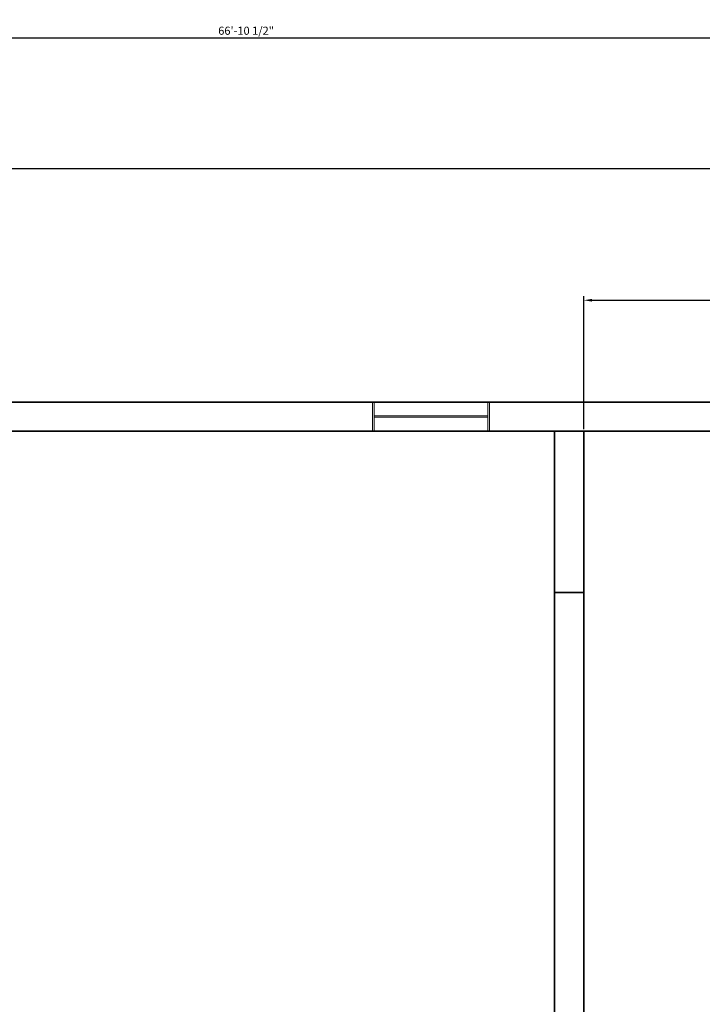
# Model space of a CAD drawing. Units: inches. Extents: x 250205121 to 250208111, y 89832590 to 89833271.
# Tile 13 of 14: x 250207599 to 250207809, y 89832955 to 89833259. Entities that reach past the tile are written whole.
import ezdxf

# ---------------------------------------------------------------- set-up
doc = ezdxf.new("R2010")
doc.units = ezdxf.units.IN
for name, color, linetype, lineweight in [('A-WALL', 7, 'Continuous', 35), ('C-PROP', 8, 'Continuous', 25), ('dimensions', 2, 'Continuous', 18), ('window', 4, 'Continuous', 18)]:
    doc.layers.add(name, color=color, linetype=linetype, lineweight=lineweight)
doc.styles.get("Standard").update_dxf_attribs({"font": 'arial.ttf'})
doc.dimstyles.new('ISO-25', dxfattribs={"dimtxt": 2.5, "dimasz": 2.5, "dimexe": 1.25, "dimexo": 0.625, "dimtad": 1, "dimlunit": 4, "dimtxsty": 'Standard', "dimcen": 2.5, "dimadec": 0, "dimazin": 0, "dimtfac": 1, "dimtmove": 0, "dimatfit": 3, "dimfxl": 1, "dimarcsym": 0})

# ---------------------------------------------------------------- blocks, each defined once
blk = doc.blocks.new('WIN-36IN')
for p, q in [((0, 0), (0, 36.08)), ((0, 36.08), (9, 36.08)), ((0, 35.58), (9, 35.58)), ((4.3, 35.58), (4.3, 0.5)), ((4.7, 35.58), (4.7, 0.5)), ((9, 36.08), (9, 0)), ((9, 0.5), (0, 0.5)), ((9, 0), (0, 0))]:
    blk.add_line(p, q)
blk = doc.blocks.new('*D66')
at = {"layer": 'Defpoints', "color": 0, "transparency": 16777216}
for p in [(250208069.71, 89833253.67), (250207267.21, 89833213.22), (250208069.71, 89833213.22)]:
    blk.add_point(p, dxfattribs=at)
at = {"layer": 'dimensions', "color": 0, "lineweight": -2, "transparency": 16777216}
for p, q in [((250207267.21, 89833213.84), (250207267.21, 89833254.92)), ((250207269.71, 89833253.67), (250208067.21, 89833253.67)), ((250208069.71, 89833213.84), (250208069.71, 89833254.92))]:
    blk.add_line(p, q, dxfattribs=at)
at = {"layer": 'dimensions', "color": 0, "transparency": 16777216}
for points in [[(250207269.71, 89833254.08), (250207269.71, 89833253.25), (250207267.21, 89833253.67)], [(250208067.21, 89833254.08), (250208067.21, 89833253.25), (250208069.71, 89833253.67)]]:
    blk.add_solid(points, dxfattribs=at)
at = {"layer": 'dimensions', "color": 0, "transparency": 16777216, "insert": (250207668.46, 89833255.58), "char_height": 2.5, "attachment_point": 5}
blk.add_mtext('66\'-10 1/2"', dxfattribs=at)
blk = doc.blocks.new('*D72')
at = {"layer": 'Defpoints', "color": 0, "transparency": 16777216}
for p in [(250207966.37, 89833172.67), (250207772.71, 89833132.22), (250207966.37, 89833132.22)]:
    blk.add_point(p, dxfattribs=at)
at = {"layer": 'dimensions', "color": 0, "lineweight": -2, "transparency": 16777216}
for p, q in [((250207772.71, 89833132.84), (250207772.71, 89833173.92)), ((250207966.37, 89833132.84), (250207966.37, 89833173.92)), ((250207775.21, 89833172.67), (250207963.87, 89833172.67))]:
    blk.add_line(p, q, dxfattribs=at)
at = {"layer": 'dimensions', "color": 0, "transparency": 16777216}
for points in [[(250207775.21, 89833173.08), (250207775.21, 89833172.25), (250207772.71, 89833172.67)], [(250207963.87, 89833173.08), (250207963.87, 89833172.25), (250207966.37, 89833172.67)]]:
    blk.add_solid(points, dxfattribs=at)
at = {"layer": 'dimensions', "color": 0, "transparency": 16777216, "insert": (250207869.54, 89833174.58), "char_height": 2.5, "attachment_point": 5}
blk.add_mtext('16\'-1 1/2"', dxfattribs=at)

msp = doc.modelspace()

# ---------------------------------------------------------------- linework, layer by layer
at = {"layer": 'A-WALL'}
for p, q in [((250207970.867, 89833141.217), (250207348.207, 89833141.217)), ((250207348.207, 89833132.217), (250207966.367, 89833132.217)), ((250207763.707, 89832721.217), (250207763.707, 89833132.217)), ((250207772.707, 89832721.217), (250207772.707, 89833132.217)), ((250207772.707, 89833082.37), (250207763.707, 89833082.37))]:
    msp.add_line(p, q, dxfattribs=at)
at = {"layer": 'C-PROP'}
msp.add_line((250208069.707, 89833213.217), (250207592.707, 89833213.217), dxfattribs=at)

# ---------------------------------------------------------------- block references
at = {"layer": 'window', "rotation": 89.99999989977422}
msp.add_blockref('WIN-36IN', (250207743.547, 89833132.217), dxfattribs=at)

# ---------------------------------------------------------------- dimensions: what is measured, and where the dimension line sits
at = {"layer": 'dimensions'}
dim = msp.add_linear_dim(base=(250208069.707, 89833253.667), p1=(250207267.207, 89833213.217), p2=(250208069.707, 89833213.217), dimstyle='ISO-25', override={"dimdec": 1, "dimlfac": 1, "dimrnd": 0, "dimzin": 1, "dimdsep": 46, "dimlunit": 4, "dimfrac": 2}, dxfattribs=at)
dim.commit()
dim.dimension.update_dxf_attribs({"geometry": '*D66', "text_midpoint": (250207668.457, 89833255.585)})
dim = msp.add_linear_dim(base=(250207966.367, 89833172.667), p1=(250207772.707, 89833132.217), p2=(250207966.367, 89833132.217), angle=0, dimstyle='ISO-25', override={"dimdec": 1, "dimlfac": 1, "dimrnd": 0, "dimzin": 1, "dimdsep": 46, "dimlunit": 4, "dimfrac": 2}, dxfattribs=at)
dim.commit()
dim.dimension.update_dxf_attribs({"geometry": '*D72', "text_midpoint": (250207869.537, 89833174.585)})

doc.saveas('drawing.dxf')
